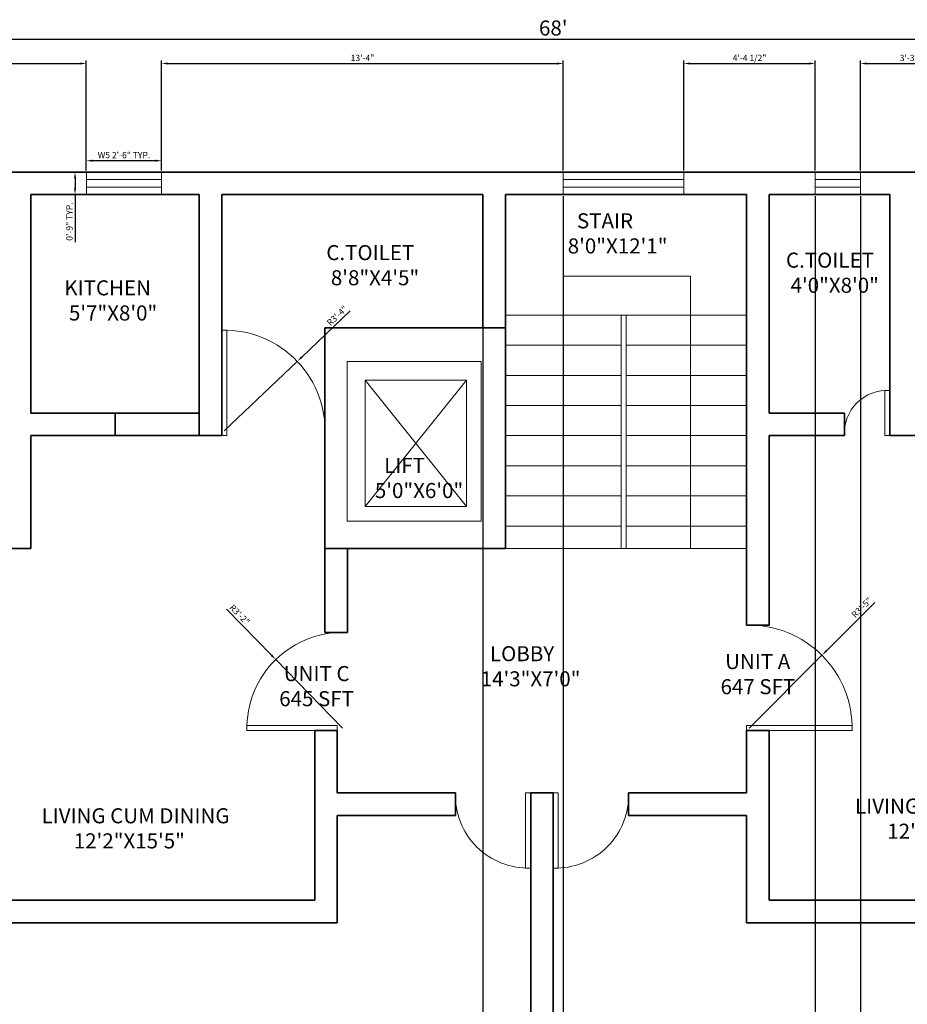
# Model space of a CAD drawing. Units: inches. Extents: x 3941 to 4852, y 2755 to 3388.
# Tile 3 of 5: x 4184 to 4537, y 2996 to 3388. Entities that reach past the tile are written whole.
import ezdxf

# ---------------------------------------------------------------- set-up
doc = ezdxf.new("R2010")
doc.units = ezdxf.units.IN
for name, color, linetype, lineweight in [('A-ANNO-DIMS', 2, 'Continuous', 18), ('A-AREA-IDEN', 7, 'Continuous', 18), ('A-DOOR', 2, 'Continuous', 18), ('A-EQPM-ELEV', 30, 'Continuous', 18), ('A-FLOR-STRS', 30, 'Continuous', 18), ('A-GLAZ', 5, 'Continuous', 18), ('A-WALL', 7, 'Continuous', 35)]:
    doc.layers.add(name, color=color, linetype=linetype, lineweight=lineweight)
doc.styles.get("Standard").update_dxf_attribs({"font": 'arial.ttf'})
doc.dimstyles.new('ISO-25', dxfattribs={"dimtxt": 2.5, "dimasz": 2.5, "dimexe": 1.25, "dimexo": 0.625, "dimtad": 1, "dimlunit": 3, "dimtxsty": 'Standard', "dimcen": 2.5, "dimadec": 0, "dimazin": 0, "dimtfac": 1, "dimtmove": 0, "dimatfit": 3, "dimfxl": 1, "dimarcsym": 0})

# ---------------------------------------------------------------- blocks, each defined once
blk = doc.blocks.new('*D1')
at = {"layer": 'A-ANNO-DIMS', "color": 0, "lineweight": -2, "transparency": 16777216}
for p, q in [((3988.25, 3328.38), (3988.25, 3381.9)), ((3990.75, 3380.65), (4801.75, 3380.65)), ((4804.25, 3328.38), (4804.25, 3381.9))]:
    blk.add_line(p, q, dxfattribs=at)
at = {"layer": 'A-ANNO-DIMS', "color": 0, "transparency": 16777216}
for points in [[(3990.75, 3381.06), (3990.75, 3380.23), (3988.25, 3380.65)], [(4801.75, 3381.06), (4801.75, 3380.23), (4804.25, 3380.65)]]:
    blk.add_solid(points, dxfattribs=at)
at = {"layer": 'Defpoints', "color": 0, "transparency": 16777216}
for p in [(4804.25, 3380.65), (3988.25, 3327.75), (4804.25, 3327.75)]:
    blk.add_point(p, dxfattribs=at)
at = {"layer": 'A-ANNO-DIMS', "color": 0, "transparency": 16777216, "insert": (4396.25, 3384.34), "char_height": 6, "attachment_point": 5}
blk.add_mtext("68'", dxfattribs=at)
blk = doc.blocks.new('WINDOW-48IN')
for p, q in [((0, 9), (0, 0)), ((0, 9), (48, 9)), ((48, 9), (48, 0)), ((0, 6), (48, 6)), ((0, 3), (48, 3)), ((48, 0), (0, 0))]:
    blk.add_line(p, q)
blk = doc.blocks.new('WINDOW-30IN')
for p, q in [((0, 0), (0, 9)), ((0, 9), (30, 9)), ((30, 9), (30, 0)), ((0, 6), (30, 6)), ((0, 3), (30, 3)), ((30, 0), (0, 0))]:
    blk.add_line(p, q)
blk = doc.blocks.new('DOOR-SWING-18IN')
for p, q in [((0.03, 0), (0.03, 2)), ((0.03, 2), (18.03, 2)), ((18.03, 0), (0.03, 0)), ((18.03, 2), (18.03, 0))]:
    blk.add_line(p, q)
blk.add_arc((17.03, 1), 17.03, 86.6335, 183.3665)
blk = doc.blocks.new('DOOR-SWING-30IN')
for p, q in [((0, 30.02), (30, 30.02)), ((0, 28.02), (0, 30.02)), ((30, 28.02), (0, 28.02)), ((30, 30.02), (30, 28.02))]:
    blk.add_line(p, q)
blk.add_arc((1, 29.02), 29.02, 268.0251, 1.9749)
blk = doc.blocks.new('*D23')
at = {"layer": 'A-ANNO-DIMS', "color": 0, "lineweight": -2, "transparency": 16777216}
for p, q in [((4210.29, 3328.38), (4210.29, 3333.5)), ((4240.29, 3328.38), (4240.29, 3333.5)), ((4237.79, 3332.25), (4212.79, 3332.25))]:
    blk.add_line(p, q, dxfattribs=at)
at = {"layer": 'A-ANNO-DIMS', "color": 0, "transparency": 16777216}
for points in [[(4212.79, 3332.67), (4212.79, 3331.84), (4210.29, 3332.25)], [(4237.79, 3332.67), (4237.79, 3331.84), (4240.29, 3332.25)]]:
    blk.add_solid(points, dxfattribs=at)
at = {"layer": 'Defpoints', "color": 0, "transparency": 16777216}
for p in [(4210.29, 3332.25), (4210.29, 3327.75), (4240.29, 3327.75)]:
    blk.add_point(p, dxfattribs=at)
at = {"layer": 'A-ANNO-DIMS', "color": 0, "transparency": 16777216, "insert": (4225.29, 3334.16), "char_height": 2.5, "attachment_point": 5}
blk.add_mtext('W5 2\'-6" TYP.', dxfattribs=at)
blk = doc.blocks.new('*D24')
at = {"layer": 'A-ANNO-DIMS', "color": 0, "lineweight": -2, "transparency": 16777216}
for p, q in [((4209.67, 3327.75), (4204.54, 3327.75)), ((4205.79, 3325.25), (4205.79, 3321.25)), ((4209.67, 3318.75), (4204.54, 3318.75)), ((4205.79, 3318.75), (4205.79, 3299.77))]:
    blk.add_line(p, q, dxfattribs=at)
at = {"layer": 'A-ANNO-DIMS', "color": 0, "transparency": 16777216}
for points in [[(4205.38, 3325.25), (4206.21, 3325.25), (4205.79, 3327.75)], [(4205.38, 3321.25), (4206.21, 3321.25), (4205.79, 3318.75)]]:
    blk.add_solid(points, dxfattribs=at)
at = {"layer": 'Defpoints', "color": 0, "transparency": 16777216}
for p in [(4210.29, 3327.75), (4205.79, 3318.75), (4210.29, 3318.75)]:
    blk.add_point(p, dxfattribs=at)
at = {"layer": 'A-ANNO-DIMS', "color": 0, "transparency": 16777216, "insert": (4203.89, 3308.01), "char_height": 2.5, "attachment_point": 5, "rotation": 90}
blk.add_mtext('0\'-9" TYP.', dxfattribs=at)
blk = doc.blocks.new('*D27')
at = {"layer": 'A-ANNO-DIMS', "color": 0, "lineweight": -2, "transparency": 16777216}
for p, q in [((4368.25, 3318.13), (4368.25, 2755.29)), ((4400.25, 3318.13), (4400.25, 2755.29)), ((4370.75, 2756.54), (4397.75, 2756.54))]:
    blk.add_line(p, q, dxfattribs=at)
at = {"layer": 'A-ANNO-DIMS', "color": 0, "transparency": 16777216}
for points in [[(4370.75, 2756.96), (4370.75, 2756.13), (4368.25, 2756.54)], [(4397.75, 2756.96), (4397.75, 2756.13), (4400.25, 2756.54)]]:
    blk.add_solid(points, dxfattribs=at)
at = {"layer": 'Defpoints', "color": 0, "transparency": 16777216}
for p in [(4368.25, 3318.75), (4400.25, 3318.75), (4400.25, 2756.54)]:
    blk.add_point(p, dxfattribs=at)
at = {"layer": 'A-ANNO-DIMS', "color": 0, "transparency": 16777216, "insert": (4384.25, 2758.44), "char_height": 2.5, "attachment_point": 5}
blk.add_mtext('2\'-8"', dxfattribs=at)
blk = doc.blocks.new('*D35')
at = {"layer": 'A-ANNO-DIMS', "color": 0, "lineweight": -2, "transparency": 16777216}
for p, q in [((4128.84, 3328.38), (4128.84, 3372.22)), ((4131.34, 3370.97), (4207.79, 3370.97)), ((4210.29, 3328.38), (4210.29, 3372.22))]:
    blk.add_line(p, q, dxfattribs=at)
at = {"layer": 'A-ANNO-DIMS', "color": 0, "transparency": 16777216}
for points in [[(4131.34, 3371.38), (4131.34, 3370.55), (4128.84, 3370.97)], [(4207.79, 3371.38), (4207.79, 3370.55), (4210.29, 3370.97)]]:
    blk.add_solid(points, dxfattribs=at)
at = {"layer": 'Defpoints', "color": 0, "transparency": 16777216}
for p in [(4210.29, 3370.97), (4128.84, 3327.75), (4210.29, 3327.75)]:
    blk.add_point(p, dxfattribs=at)
at = {"layer": 'A-ANNO-DIMS', "color": 0, "transparency": 16777216, "insert": (4169.57, 3372.88), "char_height": 2.5, "attachment_point": 5}
blk.add_mtext('6\'-9 1/2"', dxfattribs=at)
blk = doc.blocks.new('*D36')
at = {"layer": 'A-ANNO-DIMS', "color": 0, "lineweight": -2, "transparency": 16777216}
for p, q in [((4240.29, 3328.38), (4240.29, 3372.22)), ((4242.79, 3370.97), (4397.75, 3370.97)), ((4400.25, 3328.38), (4400.25, 3372.22))]:
    blk.add_line(p, q, dxfattribs=at)
at = {"layer": 'A-ANNO-DIMS', "color": 0, "transparency": 16777216}
for points in [[(4242.79, 3371.38), (4242.79, 3370.55), (4240.29, 3370.97)], [(4397.75, 3371.38), (4397.75, 3370.55), (4400.25, 3370.97)]]:
    blk.add_solid(points, dxfattribs=at)
at = {"layer": 'Defpoints', "color": 0, "transparency": 16777216}
for p in [(4400.25, 3370.97), (4240.29, 3327.75), (4400.25, 3327.75)]:
    blk.add_point(p, dxfattribs=at)
at = {"layer": 'A-ANNO-DIMS', "color": 0, "transparency": 16777216, "insert": (4320.27, 3372.87), "char_height": 2.5, "attachment_point": 5}
blk.add_mtext('13\'-4"', dxfattribs=at)
blk = doc.blocks.new('*D37')
at = {"layer": 'A-ANNO-DIMS', "color": 0, "lineweight": -2, "transparency": 16777216}
for p, q in [((4448.25, 3328.38), (4448.25, 3372.22)), ((4450.75, 3370.97), (4498.09, 3370.97)), ((4500.59, 3328.38), (4500.59, 3372.22))]:
    blk.add_line(p, q, dxfattribs=at)
at = {"layer": 'A-ANNO-DIMS', "color": 0, "transparency": 16777216}
for points in [[(4450.75, 3371.38), (4450.75, 3370.55), (4448.25, 3370.97)], [(4498.09, 3371.38), (4498.09, 3370.55), (4500.59, 3370.97)]]:
    blk.add_solid(points, dxfattribs=at)
at = {"layer": 'Defpoints', "color": 0, "transparency": 16777216}
for p in [(4500.59, 3370.97), (4448.25, 3327.75), (4500.59, 3327.75)]:
    blk.add_point(p, dxfattribs=at)
at = {"layer": 'A-ANNO-DIMS', "color": 0, "transparency": 16777216, "insert": (4474.42, 3372.88), "char_height": 2.5, "attachment_point": 5}
blk.add_mtext('4\'-4 1/2"', dxfattribs=at)
blk = doc.blocks.new('*D38')
at = {"layer": 'A-ANNO-DIMS', "color": 0, "lineweight": -2, "transparency": 16777216}
for p, q in [((4500.59, 3318.13), (4500.59, 2755.29)), ((4518.59, 3318.13), (4518.59, 2755.29)), ((4503.09, 2756.54), (4516.09, 2756.54))]:
    blk.add_line(p, q, dxfattribs=at)
at = {"layer": 'A-ANNO-DIMS', "color": 0, "transparency": 16777216}
for points in [[(4503.09, 2756.96), (4503.09, 2756.13), (4500.59, 2756.54)], [(4516.09, 2756.96), (4516.09, 2756.13), (4518.59, 2756.54)]]:
    blk.add_solid(points, dxfattribs=at)
at = {"layer": 'Defpoints', "color": 0, "transparency": 16777216}
for p in [(4500.59, 3318.75), (4518.59, 3318.75), (4518.59, 2756.54)]:
    blk.add_point(p, dxfattribs=at)
at = {"layer": 'A-ANNO-DIMS', "color": 0, "transparency": 16777216, "insert": (4509.59, 2758.44), "char_height": 2.5, "attachment_point": 5}
blk.add_mtext('1\'-6"', dxfattribs=at)
blk = doc.blocks.new('*D39')
at = {"layer": 'A-ANNO-DIMS', "color": 0, "lineweight": -2, "transparency": 16777216}
for p, q in [((4518.59, 3328.38), (4518.59, 3372.22)), ((4521.09, 3370.97), (4554.9, 3370.97)), ((4557.4, 3328.38), (4557.4, 3372.22))]:
    blk.add_line(p, q, dxfattribs=at)
at = {"layer": 'A-ANNO-DIMS', "color": 0, "transparency": 16777216}
for points in [[(4521.09, 3371.38), (4521.09, 3370.55), (4518.59, 3370.97)], [(4554.9, 3371.38), (4554.9, 3370.55), (4557.4, 3370.97)]]:
    blk.add_solid(points, dxfattribs=at)
at = {"layer": 'Defpoints', "color": 0, "transparency": 16777216}
for p in [(4557.4, 3370.97), (4518.59, 3327.75), (4557.4, 3327.75)]:
    blk.add_point(p, dxfattribs=at)
at = {"layer": 'A-ANNO-DIMS', "color": 0, "transparency": 16777216, "insert": (4538, 3372.87), "char_height": 2.5, "attachment_point": 5}
blk.add_mtext('3\'-3"', dxfattribs=at)
blk = doc.blocks.new('*D43')
at = {"layer": 'A-ANNO-DIMS', "color": 0, "lineweight": -2, "transparency": 16777216}
for p, q in [((4524.29, 3156.32), (4505.02, 3137.05)), ((4474.25, 3106.29), (4503.25, 3135.29))]:
    blk.add_line(p, q, dxfattribs=at)
at = {"layer": 'A-ANNO-DIMS', "color": 0, "transparency": 16777216}
blk.add_solid([(4504.73, 3137.35), (4505.32, 3136.76), (4503.25, 3135.29)], dxfattribs=at)
at = {"layer": 'Defpoints', "color": 0, "transparency": 16777216}
for p in [(4503.25, 3135.29), (4474.25, 3106.29)]:
    blk.add_point(p, dxfattribs=at)
at = {"layer": 'A-ANNO-DIMS', "color": 0, "transparency": 16777216, "insert": (4519.31, 3154.03), "char_height": 2.5, "attachment_point": 5, "rotation": 44.9993}
blk.add_mtext('R3\'-5"', dxfattribs=at)
blk = doc.blocks.new('*D44')
at = {"layer": 'A-ANNO-DIMS', "color": 0, "lineweight": -2, "transparency": 16777216}
for p, q in [((4315.42, 3272.49), (4296.09, 3254.06)), ((4265.25, 3224.66), (4294.28, 3252.34))]:
    blk.add_line(p, q, dxfattribs=at)
at = {"layer": 'A-ANNO-DIMS', "color": 0, "transparency": 16777216}
blk.add_solid([(4295.8, 3254.36), (4296.38, 3253.76), (4294.28, 3252.34)], dxfattribs=at)
at = {"layer": 'Defpoints', "color": 0, "transparency": 16777216}
for p in [(4294.28, 3252.34), (4265.25, 3224.66)]:
    blk.add_point(p, dxfattribs=at)
at = {"layer": 'A-ANNO-DIMS', "color": 0, "transparency": 16777216, "insert": (4310.38, 3270.32), "char_height": 2.5, "attachment_point": 5, "rotation": 43.6364}
blk.add_mtext('R3\'-4"', dxfattribs=at)
blk = doc.blocks.new('*D45')
at = {"layer": 'A-ANNO-DIMS', "color": 0, "lineweight": -2, "transparency": 16777216}
for p, q in [((4266.18, 3153.58), (4283.98, 3135.33)), ((4312.32, 3106.29), (4285.73, 3133.54))]:
    blk.add_line(p, q, dxfattribs=at)
at = {"layer": 'A-ANNO-DIMS', "color": 0, "transparency": 16777216}
blk.add_solid([(4284.28, 3135.62), (4283.68, 3135.04), (4285.73, 3133.54)], dxfattribs=at)
at = {"layer": 'Defpoints', "color": 0, "transparency": 16777216}
for p in [(4285.73, 3133.54), (4312.32, 3106.29)]:
    blk.add_point(p, dxfattribs=at)
at = {"layer": 'A-ANNO-DIMS', "color": 0, "transparency": 16777216, "insert": (4271.13, 3151.22), "char_height": 2.5, "attachment_point": 5, "rotation": 314.298}
blk.add_mtext('R3\'-2"', dxfattribs=at)

msp = doc.modelspace()

# ---------------------------------------------------------------- linework, layer by layer
at = {"layer": 'A-DOOR'}
for p, q in [((4264.254, 3222.754), (4264.254, 3264.754)), ((4264.254, 3264.754), (4266.254, 3264.754)), ((4266.254, 3264.754), (4266.254, 3222.754)), ((4266.254, 3222.754), (4264.254, 3222.754)), ((4274.254, 3105.287), (4274.254, 3107.287)), ((4274.254, 3107.287), (4310.254, 3107.287)), ((4310.254, 3107.287), (4310.254, 3105.287)), ((4515.254, 3107.287), (4473.254, 3107.287)), ((4473.254, 3107.287), (4473.254, 3105.287)), ((4515.254, 3105.287), (4515.254, 3107.287)), ((4310.254, 3105.287), (4274.254, 3105.287)), ((4473.254, 3105.287), (4515.254, 3105.287))]:
    msp.add_line(p, q, dxfattribs=at)
for centre, radius, start, end in [((4265.254, 3224.661), 40.105, 355.84337, 91.42877), ((4474.254, 3106.287), 41.012, 358.60282, 91.39718), ((4312.322, 3106.287), 38.081, 87.09216, 181.50474)]:
    msp.add_arc(centre, radius, start, end, dxfattribs=at)
at = {"layer": 'A-EQPM-ELEV'}
for p, q in [((4321.339, 3194.553), (4361.706, 3244.814)), ((4361.706, 3244.814), (4321.339, 3244.814)), ((4321.339, 3244.814), (4361.706, 3194.553))]:
    msp.add_line(p, q, dxfattribs=at)
for points in [[(4314.196, 3252.263), (4367.605, 3252.263), (4367.605, 3188.66), (4314.196, 3188.66)], [(4321.339, 3244.814), (4361.706, 3244.814), (4361.706, 3194.553), (4321.339, 3194.553)]]:
    msp.add_lwpolyline(points, close=True, dxfattribs=at)
at = {"layer": 'A-FLOR-STRS'}
for p, q in [((4400.254, 3177.754), (4400.254, 3286.335)), ((4400.254, 3286.335), (4450.933, 3286.335)), ((4450.933, 3286.335), (4450.933, 3177.754)), ((4377.254, 3270.754), (4473.254, 3270.754)), ((4377.254, 3270.754), (4473.254, 3270.754)), ((4423.254, 3177.754), (4423.254, 3270.754)), ((4425.254, 3177.754), (4425.254, 3270.754)), ((4377.254, 3258.754), (4423.254, 3258.754)), ((4425.254, 3258.754), (4473.254, 3258.754)), ((4377.254, 3246.754), (4423.254, 3246.754)), ((4425.254, 3246.754), (4473.254, 3246.754)), ((4377.254, 3234.754), (4423.254, 3234.754)), ((4425.254, 3234.754), (4473.254, 3234.754)), ((4377.254, 3222.754), (4423.254, 3222.754)), ((4425.254, 3222.754), (4473.254, 3222.754)), ((4377.254, 3210.754), (4423.254, 3210.754)), ((4425.254, 3210.754), (4473.254, 3210.754)), ((4377.254, 3198.754), (4423.254, 3198.754)), ((4425.254, 3198.754), (4473.254, 3198.754)), ((4377.254, 3186.754), (4423.254, 3186.754)), ((4425.254, 3186.754), (4473.254, 3186.754)), ((4377.254, 3177.754), (4473.254, 3177.754)), ((4377.254, 3177.754), (4473.254, 3177.754)), ((4377.254, 3177.754), (4423.254, 3177.754)), ((4423.254, 3177.754), (4400.254, 3177.754)), ((4473.254, 3177.754), (4425.254, 3177.754))]:
    msp.add_line(p, q, dxfattribs=at)
at = {"layer": 'A-GLAZ'}
for p, q in [((4500.593, 3318.754), (4500.593, 3327.754)), ((4500.593, 3327.754), (4518.593, 3327.754)), ((4518.593, 3327.754), (4518.593, 3318.754)), ((4500.593, 3324.754), (4518.593, 3324.754)), ((4500.593, 3321.754), (4518.593, 3321.754)), ((4518.593, 3318.754), (4500.593, 3318.754))]:
    msp.add_line(p, q, dxfattribs=at)
at = {"layer": 'A-WALL'}
for p, q in [((4026.254, 3327.754), (4766.254, 3327.754)), ((4188.254, 3231.754), (4188.254, 3318.754)), ((4188.254, 3318.754), (4255.254, 3318.754)), ((4255.254, 3222.754), (4255.254, 3318.754)), ((4264.254, 3222.754), (4264.254, 3318.754)), ((4264.254, 3318.754), (4368.254, 3318.754)), ((4368.254, 3265.754), (4368.254, 3318.754)), ((4377.254, 3177.754), (4377.254, 3318.754)), ((4377.254, 3318.754), (4473.254, 3318.754)), ((4473.254, 3147.287), (4473.254, 3318.754)), ((4482.254, 3231.754), (4482.254, 3318.754)), ((4482.254, 3318.754), (4530.254, 3318.754)), ((4530.254, 3222.754), (4530.254, 3318.754)), ((4305.254, 3265.754), (4377.254, 3265.754)), ((4305.254, 3177.754), (4305.254, 3265.754)), ((4188.254, 3231.754), (4255.254, 3231.754)), ((4221.754, 3231.754), (4221.754, 3222.754)), ((4482.254, 3231.754), (4512.254, 3231.754)), ((4512.254, 3222.754), (4512.254, 3231.754)), ((4188.254, 3177.754), (4188.254, 3222.754)), ((4188.254, 3222.754), (4264.254, 3222.754)), ((4482.254, 3222.754), (4512.254, 3222.754)), ((4482.254, 3147.287), (4482.254, 3222.754)), ((4530.254, 3222.754), (4604.254, 3222.754)), ((4179.254, 3177.754), (4188.254, 3177.754)), ((4305.254, 3177.754), (4377.254, 3177.754)), ((4305.254, 3177.754), (4305.254, 3144.32)), ((4314.254, 3144.32), (4314.254, 3177.754)), ((4473.254, 3147.287), (4482.254, 3147.287)), ((4305.254, 3144.32), (4314.254, 3144.32)), ((4310.254, 3105.287), (4301.254, 3105.287)), ((4301.254, 3105.287), (4301.254, 3037.754)), ((4310.254, 3080.521), (4310.254, 3105.287)), ((4473.254, 3105.287), (4482.254, 3105.287)), ((4473.254, 3080.521), (4473.254, 3105.287)), ((4482.254, 3037.754), (4482.254, 3105.287)), ((4310.254, 3080.521), (4357.254, 3080.521)), ((4357.254, 3071.521), (4357.254, 3080.521)), ((4387.254, 2906.492), (4387.254, 3080.521)), ((4387.254, 3080.521), (4396.254, 3080.521)), ((4396.254, 2906.492), (4396.254, 3080.521)), ((4426.254, 3071.521), (4426.254, 3080.521)), ((4426.254, 3080.521), (4473.254, 3080.521)), ((4310.254, 3028.754), (4310.254, 3071.521)), ((4310.254, 3071.521), (4357.254, 3071.521)), ((4426.254, 3071.521), (4473.254, 3071.521)), ((4473.254, 3028.754), (4473.254, 3071.521)), ((4301.254, 3037.754), (4154.254, 3037.754)), ((4482.254, 3037.754), (4661.254, 3037.754)), ((4310.254, 3028.754), (4154.254, 3028.754)), ((4473.254, 3028.754), (4661.254, 3028.754))]:
    msp.add_line(p, q, dxfattribs=at)

# ---------------------------------------------------------------- block references
at = {"layer": 'A-DOOR', "extrusion": (0, 0, -1), "zscale": -1}
for name, p, rotation in [('DOOR-SWING-18IN', (-4530.254, 3240.784), 269.9999999999972), ('DOOR-SWING-30IN', (-4426.27, 3080.52), 270.0000000000036)]:
    msp.add_blockref(name, p, dxfattribs=dict(at, rotation=rotation))
at = {"layer": 'A-DOOR', "rotation": 270.0000000000003}
msp.add_blockref('DOOR-SWING-30IN', (4357.237, 3080.52), dxfattribs=at)
at = {"layer": 'A-GLAZ', "rotation": 180}
for name, p in [('WINDOW-30IN', (4240.294, 3327.755)), ('WINDOW-48IN', (4448.254, 3327.755))]:
    msp.add_blockref(name, p, dxfattribs=at)

# ---------------------------------------------------------------- texts
at = {"layer": 'A-AREA-IDEN', "char_height": 6, "attachment_point": 1}
for s, width, heights, insert in [('   STAIR\\P 8\'0"X12\'1"', 69.57529, [0], (4400.181, 3311.318)), ('C.TOILET\\P 8\'8"X4\'5"', 69.57529, [0], (4305.849, 3298.649)), ('C.TOILET\\P 4\'0"X8\'0"', 69.57529, [0], (4488.93, 3295.651)), ('    KITCHEN\\P     5\'7"X8\'0"', 69.57529, [0], (4194.194, 3284.609)), ('   LIFT\\P 5\'0"X6\'0"', 69.57529, [0], (4323.379, 3213.895)), ('  LOBBY\\P14\'3"X7\'0"', 69.57529, [0], (4367.358, 3138.899)), (' UNIT A\\P647 SFT', 69.57529, [0], (4462.872, 3135.768)), (' UNIT C\\P645 SFT', 69.57529, [0], (4287.109, 3130.984)), (' LIVING CUM DINING\\P        12\'2"X15\'5"', 233.06976, [115.113], (4514.601, 3078.197)), (' LIVING CUM DINING\\P        12\'2"X15\'5"', 233.06976, [115.113], (4190.619, 3074.347))]:
    msp.add_mtext_dynamic_manual_height_columns(s, width=width, gutter_width=12.5, heights=heights, dxfattribs=dict(at, insert=insert))

# ---------------------------------------------------------------- dimensions: what is measured, and where the dimension line sits
at = {"layer": 'A-ANNO-DIMS'}
for base, p1, p2, override, picture, middle in [((4804.254, 3380.647), (3988.254, 3327.754), (4804.254, 3327.754), {"dimtxt": 6, "dimclrd": 0, "dimclre": 0, "dimclrt": 0}, '*D1', (4396.254, 3384.335)), ((4210.294, 3370.967), (4128.838, 3327.754), (4210.294, 3327.754), {"dimdec": 1, "dimlfac": 1, "dimrnd": 0, "dimzin": 1, "dimdsep": 46, "dimlunit": 4, "dimfrac": 2}, '*D35', (4169.566, 3372.884)), ((4500.593, 3370.967), (4448.254, 3327.754), (4500.593, 3327.754), {"dimdec": 1, "dimlfac": 1, "dimrnd": 0, "dimzin": 1, "dimdsep": 46, "dimlunit": 4, "dimfrac": 2}, '*D37', (4474.423, 3372.884)), ((4400.254, 3370.967), (4240.294, 3327.754), (4400.254, 3327.754), {"dimdec": 1, "dimlfac": 1, "dimrnd": 0, "dimzin": 1, "dimdsep": 46, "dimlunit": 4, "dimfrac": 2}, '*D36', (4320.274, 3372.869)), ((4557.403, 3370.967), (4518.593, 3327.754), (4557.403, 3327.754), {"dimdec": 1, "dimlfac": 1, "dimrnd": 0, "dimzin": 1, "dimdsep": 46, "dimlunit": 4, "dimfrac": 2}, '*D39', (4537.998, 3372.869)), ((4400.254, 2756.542), (4368.254, 3318.754), (4400.254, 3318.754), {"dimdec": 1, "dimlfac": 1, "dimrnd": 0, "dimzin": 1, "dimdsep": 46, "dimlunit": 4, "dimfrac": 2}, '*D27', (4384.254, 2758.443)), ((4518.593, 2756.542), (4500.593, 3318.754), (4518.593, 3318.754), {"dimdec": 1, "dimlfac": 1, "dimrnd": 0, "dimzin": 1, "dimdsep": 46, "dimlunit": 4, "dimfrac": 2}, '*D38', (4509.593, 2758.443))]:
    dim = msp.add_linear_dim(base=base, p1=p1, p2=p2, dimstyle='ISO-25', override=override, dxfattribs=at)
    dim.commit()
    dim.dimension.update_dxf_attribs({"geometry": picture, "text_midpoint": middle})
for base, p1, p2, angle, text, picture, middle in [((4210.294, 3332.254), (4240.294, 3327.754), (4210.294, 3327.754), 180, 'W5 <> TYP.', '*D23', (4225.294, 3334.156)), ((4205.794, 3318.754), (4210.294, 3327.754), (4210.294, 3318.754), 270, '<> TYP.', '*D24', (4203.892, 3308.01))]:
    dim = msp.add_linear_dim(base=base, p1=p1, p2=p2, angle=angle, text=text, dimstyle='ISO-25', override={"dimdec": 1, "dimlfac": 1, "dimrnd": 0, "dimzin": 1, "dimdsep": 46, "dimlunit": 4, "dimfrac": 2}, dxfattribs=at)
    dim.commit()
    dim.dimension.update_dxf_attribs({"geometry": picture, "text_midpoint": middle})
for center, mpoint, picture, middle in [((4265.254, 3224.661), (4294.279, 3252.337), '*D44', (4311.695, 3268.943)), ((4474.254, 3106.287), (4503.254, 3135.287), '*D43', (4520.654, 3152.687)), ((4312.322, 3106.287), (4285.726, 3133.543), '*D45', (4269.769, 3149.896))]:
    dim = msp.add_radius_dim(center=center, mpoint=mpoint, dimstyle='ISO-25', override={"dimdec": 1, "dimlfac": 1, "dimrnd": 0, "dimzin": 1, "dimdsep": 46, "dimlunit": 4, "dimfrac": 2}, dxfattribs=at)
    dim.commit()
    dim.dimension.update_dxf_attribs({"geometry": picture, "text_midpoint": middle, "dimtype": 164})

doc.saveas('drawing.dxf')
